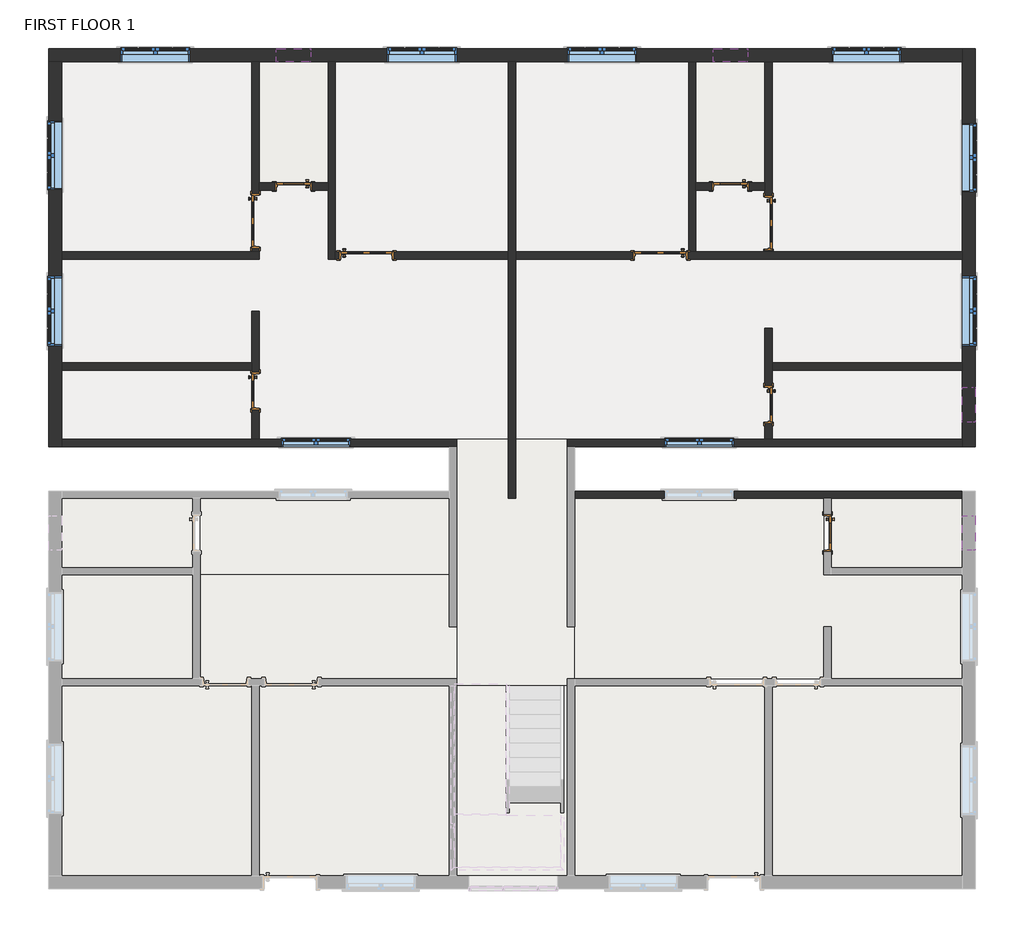
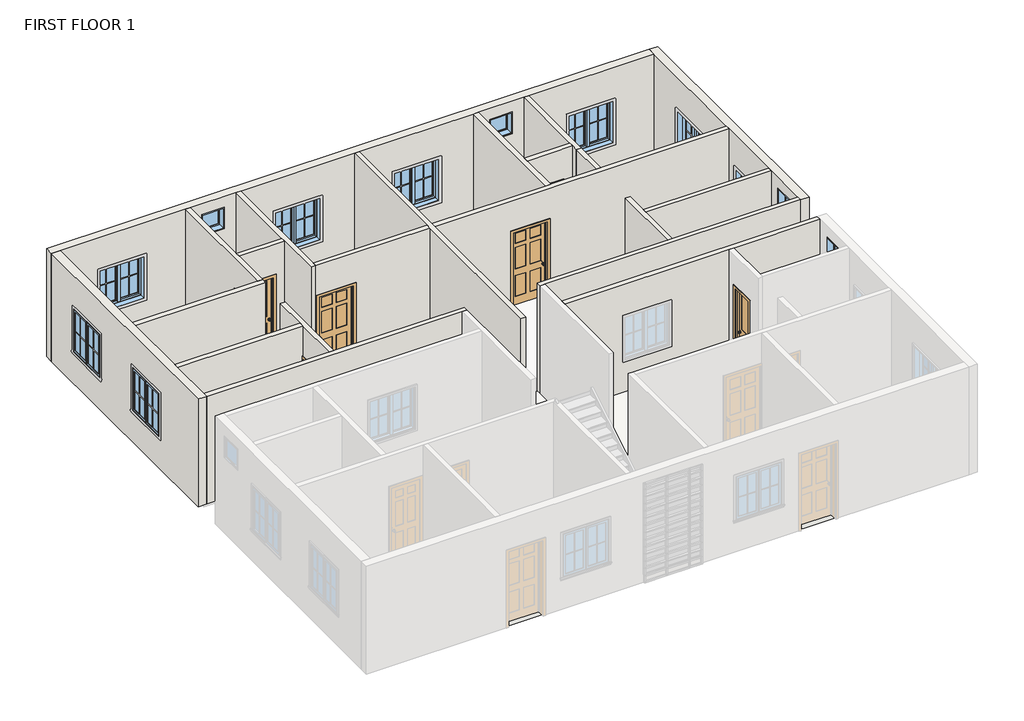
# One storey, part 3 of 4: 21 walls, 14 windows, 9 doors, 9 slabs.
"""IFC4 building model written with IfcOpenShell, lengths in millimetres."""

from ifc_helpers import new_model, si_unit, frame, origin, place, context, project, spatial, polyline, outline, extrude, faceted_brep, transform, mapped, element, save
from components import door_e337afa5, door_596d7c92, door_c610b25b, door_03e3dfb5, window_80340324, window_9200f5ac, window_c2c97eee

model = new_model("IFC4")

# Units and contexts
model_context = context("Model", 3, world=origin())
ifc_project = project(units=[si_unit("LENGTHUNIT", "METRE", prefix="MILLI")], contexts=[model_context])

# Site, building, storey
site = spatial("IfcSite", under=ifc_project)
building = spatial("IfcBuilding", under=site)
storey = spatial("IfcBuildingStorey", under=building, Name="FIRST FLOOR 1", Elevation=3200.4)

# Doors
placement = place(None, origin())
door_shape = door_e337afa5(model_context)
element("IfcDoor", 1, ObjectType="Door-Interior-Single-2_Panel-Wood : 24\" x 84\"", at=placement, inside=storey, context=model_context, shape_type="MappedRepresentation", body=[
    mapped(door_shape, transform((-8112.4137331, 4563.2156164, 3200.4), x_axis=(-1.0, 0.0, 0.0), y_axis=(0.0, -1.0, 0.0), z_axis=(0.0, 0.0, 1.0))),
])
element("IfcDoor", 2, ObjectType="Door-Interior-Single-2_Panel-Wood : 24\" x 84\"", at=placement, inside=storey, context=model_context, shape_type="MappedRepresentation", body=[
    mapped(door_shape, transform((-416.2137331, 4563.2156164, 3200.4), x_axis=(-1.0, 0.0, 0.0), y_axis=(0.0, -1.0, 0.0), z_axis=(0.0, 0.0, 1.0))),
])
element("IfcDoor", 3, ObjectType="Door-Interior-Single-2_Panel-Wood : 24\" x 84\"", at=placement, inside=storey, context=model_context, shape_type="MappedRepresentation", body=[
    mapped(door_shape, transform((-8788.6887331, 953.2406164, 3200.4), x_axis=(0.0, -1.0, 0.0), y_axis=(1.0, 0.0, 0.0), z_axis=(0.0, 0.0, 1.0))),
])
door_2_shape = door_596d7c92(model_context)
element("IfcDoor", 4, ObjectType="Door-Interior-Single-2_Panel-Wood : 24\" x 84\"", at=placement, inside=storey, context=model_context, shape_type="MappedRepresentation", body=[
    mapped(door_2_shape, transform((260.0612669, 711.9406164, 3200.4), x_axis=(0.0, -1.0, 0.0), y_axis=(1.0, 0.0, 0.0), z_axis=(0.0, 0.0, 1.0))),
])
element("IfcDoor", 5, ObjectType="Door-Interior-Single-2_Panel-Wood : 24\" x 84\"", at=placement, inside=storey, context=model_context, shape_type="MappedRepresentation", body=[
    mapped(door_2_shape, transform((1301.4612669, -1548.6593836, 3200.4), x_axis=(0.0, -1.0, 0.0), y_axis=(1.0, 0.0, 0.0), z_axis=(0.0, 0.0, 1.0))),
])
door_3_shape = door_c610b25b(model_context)
element("IfcDoor", 6, ObjectType="Door-Interior-Single-6_Panel-Wood : 36\" x 84\"", at=placement, inside=storey, context=model_context, shape_type="MappedRepresentation", body=[
    mapped(door_3_shape, transform((-8788.6887331, 3950.4406164, 3200.4), x_axis=(0.0, -1.0, 0.0), y_axis=(1.0, 0.0, 0.0), z_axis=(0.0, 0.0, 1.0))),
])
element("IfcDoor", 7, ObjectType="Door-Interior-Single-6_Panel-Wood : 36\" x 84\"", at=placement, inside=storey, context=model_context, shape_type="MappedRepresentation", body=[
    mapped(door_3_shape, transform((-1648.1137331, 3344.0156164, 3200.4), x_axis=(-1.0, 0.0, 0.0), y_axis=(0.0, -1.0, 0.0), z_axis=(0.0, 0.0, 1.0))),
])
door_4_shape = door_03e3dfb5(model_context)
element("IfcDoor", 8, ObjectType="Door-Interior-Single-6_Panel-Wood : 36\" x 84\"", at=placement, inside=storey, context=model_context, shape_type="MappedRepresentation", body=[
    mapped(door_4_shape, transform((-6829.7137331, 3344.0156164, 3200.4), x_axis=(1.0, 0.0, 0.0), y_axis=(0.0, 1.0, 0.0), z_axis=(0.0, 0.0, 1.0))),
])
element("IfcDoor", 9, ObjectType="Door-Interior-Single-6_Panel-Wood : 36\" x 84\"", at=placement, inside=storey, context=model_context, shape_type="MappedRepresentation", body=[
    mapped(door_4_shape, transform((260.0612669, 3912.3406164, 3200.4), x_axis=(0.0, -1.0, 0.0), y_axis=(1.0, 0.0, 0.0), z_axis=(0.0, 0.0, 1.0))),
])

# Slabs
element("IfcSlab", 10, ObjectType="marble tiles", at=placement, inside=storey, context=model_context, shape_type="SweptSolid", body=[
    extrude(outline(polyline([(-9890.4137331, -939.0593836), (-9890.4137331, -2158.2593836), (-12201.8137331, -2158.2593836), (-12201.8137331, -939.0593836), (-9890.4137331, -939.0593836)])), frame((0.0, 0.0, 3048.0), z_axis=(0.0, 0.0, 1.0), x_axis=(1.0, 0.0, 0.0)), (0.0, 0.0, 1.0), 152.4),
    extrude(outline(polyline([(3673.1862669, -2158.2593836), (1361.7862669, -2158.2593836), (1361.7862669, -939.0593836), (3673.1862669, -939.0593836), (3673.1862669, -2158.2593836)])), frame((0.0, 0.0, 3048.0), z_axis=(0.0, 0.0, 1.0), x_axis=(1.0, 0.0, 0.0)), (0.0, 0.0, 1.0), 152.4),
    extrude(outline(polyline([(-7502.8137331, 6758.7281164), (-7502.8137331, 4623.5406164), (-8722.0137331, 4623.5406164), (-8722.0137331, 6758.7281164), (-7502.8137331, 6758.7281164)])), frame((0.0, 0.0, 3048.0), z_axis=(0.0, 0.0, 1.0), x_axis=(1.0, 0.0, 0.0)), (0.0, 0.0, 1.0), 152.4),
    extrude(outline(polyline([(193.3862669, 4623.5406164), (-1025.8137331, 4623.5406164), (-1025.8137331, 6758.7281164), (193.3862669, 6758.7281164), (193.3862669, 4623.5406164)])), frame((0.0, 0.0, 3048.0), z_axis=(0.0, 0.0, 1.0), x_axis=(1.0, 0.0, 0.0)), (0.0, 0.0, 1.0), 152.4),
])
element("IfcSlab", 11, ObjectType="marble tiles", at=placement, inside=storey, context=model_context, shape_type="SweptSolid", body=[
    extrude(outline(polyline([(-5242.2137331, -7593.8593836), (-12201.8137331, -7593.8593836), (-12201.8137331, -2285.2593836), (-5242.2137331, -2285.2593836), (-5242.2137331, -7593.8593836)])), frame((0.0, 0.0, 3048.0), z_axis=(0.0, 0.0, 1.0), x_axis=(1.0, 0.0, 0.0)), (0.0, 0.0, 1.0), 152.4),
])
element("IfcSlab", 12, ObjectType="marble tiles", at=placement, inside=storey, context=model_context, shape_type="SweptSolid", body=[
    extrude(outline(polyline([(-5242.2137331, -2285.2593836), (-9763.4137331, -2285.2593836), (-9763.4137331, -812.0593836), (-5242.2137331, -812.0593836), (-5242.2137331, -2285.2593836)])), frame((0.0, 0.0, 3048.0), z_axis=(0.0, 0.0, 1.0), x_axis=(1.0, 0.0, 0.0)), (0.0, 0.0, 1.0), 152.4),
])
element("IfcSlab", 13, ObjectType="marble tiles", at=placement, inside=storey, context=model_context, shape_type="SweptSolid", body=[
    extrude(outline(polyline([(-3159.4137331, -4241.0593836), (-5242.2137331, -4241.0593836), (-5242.2137331, 102.3406164), (-3159.4137331, 102.3406164), (-3159.4137331, -4241.0593836)])), frame((0.0, 0.0, 3048.0), z_axis=(0.0, 0.0, 1.0), x_axis=(1.0, 0.0, 0.0)), (0.0, 0.0, 1.0), 152.4),
])
element("IfcSlab", 14, ObjectType="marble tiles", at=placement, inside=storey, context=model_context, shape_type="SweptSolid", body=[
    extrude(outline(polyline([(-3286.4137331, -7593.8593836), (-5242.2137331, -7593.8593836), (-5242.2137331, -4241.0593836), (-3286.4137331, -4241.0593836), (-3286.4137331, -7593.8593836)])), frame((0.0, 0.0, 3048.0), z_axis=(0.0, 0.0, 1.0), x_axis=(1.0, 0.0, 0.0)), (0.0, 0.0, 1.0), 152.4),
    extrude(outline(polyline([(193.3862669, -7593.8593836), (-3159.4137331, -7593.8593836), (-3159.4137331, -4241.0593836), (193.3862669, -4241.0593836), (193.3862669, -7593.8593836)])), frame((0.0, 0.0, 3048.0), z_axis=(0.0, 0.0, 1.0), x_axis=(1.0, 0.0, 0.0)), (0.0, 0.0, 1.0), 152.4),
    extrude(outline(polyline([(3673.1862669, -7593.8593836), (320.3862669, -7593.8593836), (320.3862669, -4241.0593836), (3673.1862669, -4241.0593836), (3673.1862669, -7593.8593836)])), frame((0.0, 0.0, 3048.0), z_axis=(0.0, 0.0, 1.0), x_axis=(1.0, 0.0, 0.0)), (0.0, 0.0, 1.0), 152.4),
    extrude(outline(polyline([(1234.7862669, -4114.0593836), (-3159.4137331, -4114.0593836), (-3159.4137331, -939.0593836), (1234.7862669, -939.0593836), (1234.7862669, -2285.2593836), (3673.1862669, -2285.2593836), (3673.1862669, -4114.0593836), (1234.7862669, -4114.0593836)])), frame((0.0, 0.0, 3048.0), z_axis=(0.0, 0.0, 1.0), x_axis=(1.0, 0.0, 0.0)), (0.0, 0.0, 1.0), 152.4),
])
element("IfcSlab", 15, ObjectType="marble tiles", at=placement, inside=storey, context=model_context, shape_type="SweptSolid", body=[
    extrude(outline(polyline([(-5242.2137331, -7593.8593836), (-12201.8137331, -7593.8593836), (-12201.8137331, -2285.2593836), (-5242.2137331, -2285.2593836), (-5242.2137331, -7593.8593836)])), frame((0.0, 0.0, 3048.0), z_axis=(0.0, 0.0, 1.0), x_axis=(1.0, 0.0, 0.0)), (0.0, 0.0, 1.0), 152.4),
])
element("IfcSlab", 16, ObjectType="marble tiles", at=placement, inside=storey, context=model_context, shape_type="SweptSolid", body=[
    extrude(outline(polyline([(-5242.2137331, -2285.2593836), (-9763.4137331, -2285.2593836), (-9763.4137331, -812.0593836), (-5242.2137331, -812.0593836), (-5242.2137331, -2285.2593836)])), frame((0.0, 0.0, 3048.0), z_axis=(0.0, 0.0, 1.0), x_axis=(1.0, 0.0, 0.0)), (0.0, 0.0, 1.0), 152.4),
])
element("IfcSlab", 17, ObjectType="marble tiles", at=placement, inside=storey, context=model_context, shape_type="SweptSolid", body=[
    extrude(outline(polyline([(-3159.4137331, -4241.0593836), (-5242.2137331, -4241.0593836), (-5242.2137331, 102.3406164), (-3159.4137331, 102.3406164), (-3159.4137331, -4241.0593836)])), frame((0.0, 0.0, 3048.0), z_axis=(0.0, 0.0, 1.0), x_axis=(1.0, 0.0, 0.0)), (0.0, 0.0, 1.0), 152.4),
])
element("IfcSlab", 18, ObjectType="marble tiles", at=placement, inside=storey, context=model_context, shape_type="SweptSolid", body=[
    extrude(outline(polyline([(-3286.4137331, -7593.8593836), (-5242.2137331, -7593.8593836), (-5242.2137331, -4241.0593836), (-3286.4137331, -4241.0593836), (-3286.4137331, -7593.8593836)])), frame((0.0, 0.0, 3048.0), z_axis=(0.0, 0.0, 1.0), x_axis=(1.0, 0.0, 0.0)), (0.0, 0.0, 1.0), 152.4),
    extrude(outline(polyline([(193.3862669, -7593.8593836), (-3159.4137331, -7593.8593836), (-3159.4137331, -4241.0593836), (193.3862669, -4241.0593836), (193.3862669, -7593.8593836)])), frame((0.0, 0.0, 3048.0), z_axis=(0.0, 0.0, 1.0), x_axis=(1.0, 0.0, 0.0)), (0.0, 0.0, 1.0), 152.4),
    extrude(outline(polyline([(3673.1862669, -7593.8593836), (320.3862669, -7593.8593836), (320.3862669, -4241.0593836), (3673.1862669, -4241.0593836), (3673.1862669, -7593.8593836)])), frame((0.0, 0.0, 3048.0), z_axis=(0.0, 0.0, 1.0), x_axis=(1.0, 0.0, 0.0)), (0.0, 0.0, 1.0), 152.4),
    extrude(outline(polyline([(1234.7862669, -4114.0593836), (-3159.4137331, -4114.0593836), (-3159.4137331, -939.0593836), (1234.7862669, -939.0593836), (1234.7862669, -2285.2593836), (3673.1862669, -2285.2593836), (3673.1862669, -4114.0593836), (1234.7862669, -4114.0593836)])), frame((0.0, 0.0, 3048.0), z_axis=(0.0, 0.0, 1.0), x_axis=(1.0, 0.0, 0.0)), (0.0, 0.0, 1.0), 152.4),
])

# Walls
element("IfcWall", 19, ObjectType="Inner Wall 5\"", at=placement, inside=storey, context=model_context, shape_type="Brep", body=[
    faceted_brep([(-12201.8137331, -24.6593836, 3200.4), (-5369.2137331, -24.6593836, 3200.4), (-5242.2137331, -24.6593836, 3200.4), (-5242.2137331, -24.6593836, 6248.4), (-5369.2137331, -24.6593836, 6248.4), (-12201.8137331, -24.6593836, 6248.4), (-7109.1137331, -24.6593836, 5334.0), (-7109.1137331, -24.6593836, 4114.8), (-8328.3137331, -24.6593836, 4114.8), (-8328.3137331, -24.6593836, 5334.0), (-12201.8137331, 102.3406164, 3200.4), (-12201.8137331, 102.3406164, 6248.4), (-8849.0137331, 102.3406164, 6248.4), (-8722.0137331, 102.3406164, 6248.4), (-5242.2137331, 102.3406164, 6248.4), (-5242.2137331, 102.3406164, 3200.4), (-8722.0137331, 102.3406164, 3200.4), (-8849.0137331, 102.3406164, 3200.4), (-7109.1137331, 102.3406164, 5334.0), (-8328.3137331, 102.3406164, 5334.0), (-8328.3137331, 102.3406164, 4114.8), (-7109.1137331, 102.3406164, 4114.8)], [[[0, 1, 2, 3, 4, 5], [6, 7, 8, 9]], [[10, 11, 12, 13, 14, 15, 16, 17], [18, 19, 20, 21]], [[2, 1, 0, 10, 17, 16, 15]], [[5, 4, 3, 14, 13, 12, 11]], [[0, 5, 11, 10]], [[3, 2, 15, 14]], [[7, 6, 18, 21]], [[8, 7, 21, 20]], [[9, 8, 20, 19]], [[6, 9, 19, 18]]]),
])
element("IfcWall", 20, ObjectType="Inner Wall 5\"", at=placement, inside=storey, context=model_context, shape_type="Brep", body=[
    faceted_brep([(3673.1862669, 102.3406164, 3200.4), (320.3862669, 102.3406164, 3200.4), (193.3862669, 102.3406164, 3200.4), (-3286.4137331, 102.3406164, 3200.4), (-3286.4137331, 102.3406164, 6248.4), (193.3862669, 102.3406164, 6248.4), (320.3862669, 102.3406164, 6248.4), (3673.1862669, 102.3406164, 6248.4), (-352.7137331, 102.3406164, 5334.0), (-1571.9137331, 102.3406164, 5334.0), (-1571.9137331, 102.3406164, 4114.8), (-352.7137331, 102.3406164, 4114.8), (3673.1862669, -24.6593836, 3200.4), (3673.1862669, -24.6593836, 6248.4), (-3159.4137331, -24.6593836, 6248.4), (-3286.4137331, -24.6593836, 6248.4), (-3286.4137331, -24.6593836, 3200.4), (-3159.4137331, -24.6593836, 3200.4), (-352.7137331, -24.6593836, 5334.0), (-352.7137331, -24.6593836, 4114.8), (-1571.9137331, -24.6593836, 4114.8), (-1571.9137331, -24.6593836, 5334.0)], [[[0, 1, 2, 3, 4, 5, 6, 7], [8, 9, 10, 11]], [[12, 13, 14, 15, 16, 17], [18, 19, 20, 21]], [[3, 2, 1, 0, 12, 17, 16]], [[7, 6, 5, 4, 15, 14, 13]], [[0, 7, 13, 12]], [[4, 3, 16, 15]], [[19, 18, 8, 11]], [[20, 19, 11, 10]], [[21, 20, 10, 9]], [[18, 21, 9, 8]]]),
])
element("IfcWall", 21, ObjectType="Inner Wall 5\"", at=placement, inside=storey, context=model_context, shape_type="Brep", body=[
    faceted_brep([(3673.1862669, -812.0593836, 3200.4), (-3159.4137331, -812.0593836, 3200.4), (-3159.4137331, -812.0593836, 6248.4), (3673.1862669, -812.0593836, 6248.4), (-352.7137331, -812.0593836, 5334.0), (-1571.9137331, -812.0593836, 5334.0), (-1571.9137331, -812.0593836, 4114.8), (-352.7137331, -812.0593836, 4114.8), (3673.1862669, -939.0593836, 3200.4), (3673.1862669, -939.0593836, 6248.4), (1361.7862669, -939.0593836, 6248.4), (1234.7862669, -939.0593836, 6248.4), (-3159.4137331, -939.0593836, 6248.4), (-3159.4137331, -939.0593836, 3200.4), (1234.7862669, -939.0593836, 3200.4), (1361.7862669, -939.0593836, 3200.4), (-352.7137331, -939.0593836, 5334.0), (-352.7137331, -939.0593836, 4114.8), (-1571.9137331, -939.0593836, 4114.8), (-1571.9137331, -939.0593836, 5334.0)], [[[0, 1, 2, 3], [4, 5, 6, 7]], [[8, 9, 10, 11, 12, 13, 14, 15], [16, 17, 18, 19]], [[1, 0, 8, 15, 14, 13]], [[3, 2, 12, 11, 10, 9]], [[0, 3, 9, 8]], [[2, 1, 13, 12]], [[17, 16, 4, 7]], [[18, 17, 7, 6]], [[19, 18, 6, 5]], [[16, 19, 5, 4]]]),
])
element("IfcWall", 22, ObjectType="Inner Wall 5\"", at=placement, inside=storey, context=model_context, shape_type="Brep", body=[
    faceted_brep([(-12201.8137331, 3277.3406164, 3200.4), (-8722.0137331, 3277.3406164, 3200.4), (-8722.0137331, 3277.3406164, 6248.4), (-12201.8137331, 3277.3406164, 6248.4), (-12201.8137331, 3404.3406164, 3200.4), (-12201.8137331, 3404.3406164, 6248.4), (-8849.0137331, 3404.3406164, 6248.4), (-8722.0137331, 3404.3406164, 6248.4), (-8722.0137331, 3404.3406164, 3200.4), (-8849.0137331, 3404.3406164, 3200.4)], [[[0, 1, 2, 3]], [[4, 5, 6, 7, 8, 9]], [[1, 0, 4, 9, 8]], [[3, 2, 7, 6, 5]], [[0, 3, 5, 4]], [[2, 1, 8, 7]]]),
])
element("IfcWall", 23, ObjectType="Inner Wall 5\"", at=placement, inside=storey, context=model_context, shape_type="Brep", body=[
    faceted_brep([(-8722.0137331, 6758.7281164, 6248.4), (-8722.0137331, 4623.5406164, 6248.4), (-8722.0137331, 4496.5406164, 6248.4), (-8722.0137331, 3404.3406164, 6248.4), (-8722.0137331, 3404.3406164, 3200.4), (-8722.0137331, 3467.8406164, 3200.4), (-8722.0137331, 3467.8406164, 5359.4), (-8722.0137331, 4433.0406164, 5359.4), (-8722.0137331, 4433.0406164, 3200.4), (-8722.0137331, 4496.5406164, 3200.4), (-8722.0137331, 4623.5406164, 3200.4), (-8722.0137331, 6758.7281164, 3200.4), (-8849.0137331, 3404.3406164, 6248.4), (-8849.0137331, 6758.7281164, 6248.4), (-8849.0137331, 6758.7281164, 3200.4), (-8849.0137331, 4433.0406164, 3200.4), (-8849.0137331, 4433.0406164, 5359.4), (-8849.0137331, 3467.8406164, 5359.4), (-8849.0137331, 3467.8406164, 3200.4), (-8849.0137331, 3404.3406164, 3200.4)], [[[0, 1, 2, 3, 4, 5, 6, 7, 8, 9, 10, 11]], [[12, 13, 14, 15, 16, 17, 18, 19]], [[4, 19, 18, 5]], [[14, 11, 10, 9, 8, 15]], [[3, 2, 1, 0, 13, 12]], [[4, 3, 12, 19]], [[0, 11, 14, 13]], [[17, 6, 5, 18]], [[6, 17, 16, 7]], [[7, 16, 15, 8]]]),
])
element("IfcWall", 24, ObjectType="Inner Wall 5\"", at=placement, inside=storey, context=model_context, shape_type="SweptSolid", body=[
    extrude(outline(polyline([(6248.4, -7502.8137331), (6248.4, -8722.0137331), (3200.4, -8722.0137331), (3200.4, -8442.6137331), (5359.4, -8442.6137331), (5359.4, -7782.2137331), (3200.4, -7782.2137331), (3200.4, -7502.8137331), (6248.4, -7502.8137331)])), frame((0.0, 4496.5406164, 0.0), z_axis=(0.0, 1.0, 0.0), x_axis=(0.0, 0.0, 1.0)), (0.0, 0.0, 1.0), 127.0),
])
element("IfcWall", 25, ObjectType="Inner Wall 5\"", at=placement, inside=storey, context=model_context, shape_type="Brep", body=[
    faceted_brep([(-7375.8137331, 3277.3406164, 3200.4), (-7375.8137331, 3404.3406164, 3200.4), (-7375.8137331, 6758.7281164, 3200.4), (-7375.8137331, 6758.7281164, 6248.4), (-7375.8137331, 3404.3406164, 6248.4), (-7375.8137331, 3277.3406164, 6248.4), (-7502.8137331, 3277.3406164, 3200.4), (-7502.8137331, 3277.3406164, 6248.4), (-7502.8137331, 4496.5406164, 6248.4), (-7502.8137331, 4623.5406164, 6248.4), (-7502.8137331, 6758.7281164, 6248.4), (-7502.8137331, 6758.7281164, 3200.4), (-7502.8137331, 4623.5406164, 3200.4), (-7502.8137331, 4496.5406164, 3200.4)], [[[0, 1, 2, 3, 4, 5]], [[6, 7, 8, 9, 10, 11, 12, 13]], [[2, 1, 0, 6, 13, 12, 11]], [[5, 4, 3, 10, 9, 8, 7]], [[3, 2, 11, 10]], [[0, 5, 7, 6]]]),
])
element("IfcWall", 26, ObjectType="Inner Wall 5\"", at=placement, inside=storey, context=model_context, shape_type="Brep", body=[
    faceted_brep([(-4327.8137331, 6758.7281164, 3200.4), (-4327.8137331, 3404.3406164, 3200.4), (-4327.8137331, 3277.3406164, 3200.4), (-4327.8137331, -939.0593836, 3200.4), (-4327.8137331, -939.0593836, 6248.4), (-4327.8137331, 3277.3406164, 6248.4), (-4327.8137331, 3404.3406164, 6248.4), (-4327.8137331, 6758.7281164, 6248.4), (-4200.8137331, 6758.7281164, 3200.4), (-4200.8137331, 6758.7281164, 6248.4), (-4200.8137331, 3404.3406164, 6248.4), (-4200.8137331, 3277.3406164, 6248.4), (-4200.8137331, -939.0593836, 6248.4), (-4200.8137331, -939.0593836, 3200.4), (-4200.8137331, 3277.3406164, 3200.4), (-4200.8137331, 3404.3406164, 3200.4)], [[[0, 1, 2, 3, 4, 5, 6, 7]], [[8, 9, 10, 11, 12, 13, 14, 15]], [[3, 2, 1, 0, 8, 15, 14, 13]], [[4, 3, 13, 12]], [[7, 6, 5, 4, 12, 11, 10, 9]], [[0, 7, 9, 8]]]),
])
element("IfcWall", 27, ObjectType="Inner Wall 5\"", at=placement, inside=storey, context=model_context, shape_type="SweptSolid", body=[
    extrude(outline(polyline([(6248.4, -4327.8137331), (6248.4, -7375.8137331), (3200.4, -7375.8137331), (3200.4, -7312.3137331), (5359.4, -7312.3137331), (5359.4, -6347.1137331), (3200.4, -6347.1137331), (3200.4, -4327.8137331), (6248.4, -4327.8137331)])), frame((0.0, 3277.3406164, 0.0), z_axis=(0.0, 1.0, 0.0), x_axis=(0.0, 0.0, 1.0)), (0.0, 0.0, 1.0), 127.0),
])
element("IfcWall", 28, ObjectType="Inner Wall 5\"", at=placement, inside=storey, context=model_context, shape_type="Brep", body=[
    faceted_brep([(3673.1862669, 3277.3406164, 6248.4), (-4200.8137331, 3277.3406164, 6248.4), (-4200.8137331, 3277.3406164, 3200.4), (-2130.7137331, 3277.3406164, 3200.4), (-2130.7137331, 3277.3406164, 5359.4), (-1165.5137331, 3277.3406164, 5359.4), (-1165.5137331, 3277.3406164, 3200.4), (3673.1862669, 3277.3406164, 3200.4), (-4200.8137331, 3404.3406164, 6248.4), (-1152.8137331, 3404.3406164, 6248.4), (-1025.8137331, 3404.3406164, 6248.4), (193.3862669, 3404.3406164, 6248.4), (320.3862669, 3404.3406164, 6248.4), (3673.1862669, 3404.3406164, 6248.4), (3673.1862669, 3404.3406164, 3200.4), (320.3862669, 3404.3406164, 3200.4), (193.3862669, 3404.3406164, 3200.4), (-1025.8137331, 3404.3406164, 3200.4), (-1152.8137331, 3404.3406164, 3200.4), (-1165.5137331, 3404.3406164, 3200.4), (-1165.5137331, 3404.3406164, 5359.4), (-2130.7137331, 3404.3406164, 5359.4), (-2130.7137331, 3404.3406164, 3200.4), (-4200.8137331, 3404.3406164, 3200.4)], [[[0, 1, 2, 3, 4, 5, 6, 7]], [[8, 9, 10, 11, 12, 13, 14, 15, 16, 17, 18, 19, 20, 21, 22, 23]], [[2, 23, 22, 3]], [[14, 7, 6, 19, 18, 17, 16, 15]], [[1, 0, 13, 12, 11, 10, 9, 8]], [[2, 1, 8, 23]], [[0, 7, 14, 13]], [[21, 4, 3, 22]], [[4, 21, 20, 5]], [[5, 20, 19, 6]]]),
])
element("IfcWall", 29, ObjectType="Inner Wall 5\"", at=placement, inside=storey, context=model_context, shape_type="Brep", body=[
    faceted_brep([(-1025.8137331, 3404.3406164, 3200.4), (-1025.8137331, 4496.5406164, 3200.4), (-1025.8137331, 4623.5406164, 3200.4), (-1025.8137331, 6758.7281164, 3200.4), (-1025.8137331, 6758.7281164, 6248.4), (-1025.8137331, 4623.5406164, 6248.4), (-1025.8137331, 4496.5406164, 6248.4), (-1025.8137331, 3404.3406164, 6248.4), (-1152.8137331, 3404.3406164, 3200.4), (-1152.8137331, 3404.3406164, 6248.4), (-1152.8137331, 6758.7281164, 6248.4), (-1152.8137331, 6758.7281164, 3200.4)], [[[0, 1, 2, 3, 4, 5, 6, 7]], [[8, 9, 10, 11]], [[3, 2, 1, 0, 8, 11]], [[7, 6, 5, 4, 10, 9]], [[0, 7, 9, 8]], [[4, 3, 11, 10]]]),
])
element("IfcWall", 30, ObjectType="Inner Wall 5\"", at=placement, inside=storey, context=model_context, shape_type="SweptSolid", body=[
    extrude(outline(polyline([(6248.4, 193.3862669), (6248.4, -1025.8137331), (3200.4, -1025.8137331), (3200.4, -746.4137331), (5359.4, -746.4137331), (5359.4, -86.0137331), (3200.4, -86.0137331), (3200.4, 193.3862669), (6248.4, 193.3862669)])), frame((0.0, 4496.5406164, 0.0), z_axis=(0.0, 1.0, 0.0), x_axis=(0.0, 0.0, 1.0)), (0.0, 0.0, 1.0), 127.0),
])
element("IfcWall", 31, ObjectType="Inner Wall 5\"", at=placement, inside=storey, context=model_context, shape_type="Brep", body=[
    faceted_brep([(320.3862669, 6758.7281164, 6248.4), (320.3862669, 4318.7406164, 6248.4), (320.3862669, 4318.7406164, 5359.4), (320.3862669, 4394.9406164, 5359.4), (320.3862669, 4394.9406164, 3200.4), (320.3862669, 6758.7281164, 3200.4), (193.3862669, 4318.7406164, 6248.4), (193.3862669, 4496.5406164, 6248.4), (193.3862669, 4623.5406164, 6248.4), (193.3862669, 6758.7281164, 6248.4), (193.3862669, 6758.7281164, 3200.4), (193.3862669, 4623.5406164, 3200.4), (193.3862669, 4496.5406164, 3200.4), (193.3862669, 4394.9406164, 3200.4), (193.3862669, 4394.9406164, 5359.4), (193.3862669, 4318.7406164, 5359.4)], [[[0, 1, 2, 3, 4, 5]], [[6, 7, 8, 9, 10, 11, 12, 13, 14, 15]], [[10, 5, 4, 13, 12, 11]], [[1, 0, 9, 8, 7, 6]], [[1, 6, 15, 2]], [[0, 5, 10, 9]], [[14, 3, 2, 15]], [[3, 14, 13, 4]]]),
])
element("IfcWall", 32, ObjectType="Inner Wall 5\"", at=placement, inside=storey, context=model_context, shape_type="SweptSolid", body=[
    extrude(outline(polyline([(320.3862669, 1448.5406164), (3673.1862669, 1448.5406164), (3673.1862669, 1321.5406164), (320.3862669, 1321.5406164), (320.3862669, 1448.5406164)])), frame((0.0, 0.0, 3200.4), z_axis=(0.0, 0.0, 1.0), x_axis=(1.0, 0.0, 0.0)), (0.0, 0.0, 1.0), 3048.0),
])
element("IfcWall", 33, ObjectType="Inner Wall 5\"", at=placement, inside=storey, context=model_context, shape_type="Brep", body=[
    faceted_brep([(193.3862669, 102.3406164, 6248.4), (193.3862669, 2058.1406164, 6248.4), (193.3862669, 2058.1406164, 3200.4), (193.3862669, 1042.1406164, 3200.4), (193.3862669, 1042.1406164, 5359.4), (193.3862669, 381.7406164, 5359.4), (193.3862669, 381.7406164, 3200.4), (193.3862669, 102.3406164, 3200.4), (320.3862669, 2058.1406164, 6248.4), (320.3862669, 1448.5406164, 6248.4), (320.3862669, 1321.5406164, 6248.4), (320.3862669, 102.3406164, 6248.4), (320.3862669, 102.3406164, 3200.4), (320.3862669, 381.7406164, 3200.4), (320.3862669, 381.7406164, 5359.4), (320.3862669, 1042.1406164, 5359.4), (320.3862669, 1042.1406164, 3200.4), (320.3862669, 1321.5406164, 3200.4), (320.3862669, 1448.5406164, 3200.4), (320.3862669, 2058.1406164, 3200.4)], [[[0, 1, 2, 3, 4, 5, 6, 7]], [[8, 9, 10, 11, 12, 13, 14, 15, 16, 17, 18, 19]], [[2, 19, 18, 17, 16, 3]], [[12, 7, 6, 13]], [[1, 0, 11, 10, 9, 8]], [[2, 1, 8, 19]], [[0, 7, 12, 11]], [[5, 14, 13, 6]], [[14, 5, 4, 15]], [[15, 4, 3, 16]]]),
])
element("IfcWall", 34, ObjectType="Inner Wall 5\"", at=placement, inside=storey, context=model_context, shape_type="Brep", body=[
    faceted_brep([(-8722.0137331, 2362.9406164, 3200.4), (-8722.0137331, 2362.9406164, 6248.4), (-8722.0137331, 102.3406164, 6248.4), (-8722.0137331, 102.3406164, 3200.4), (-8722.0137331, 623.0406164, 3200.4), (-8722.0137331, 623.0406164, 5359.4), (-8722.0137331, 1283.4406164, 5359.4), (-8722.0137331, 1283.4406164, 3200.4), (-8849.0137331, 2362.9406164, 6248.4), (-8849.0137331, 2362.9406164, 3200.4), (-8849.0137331, 1448.5406164, 3200.4), (-8849.0137331, 1321.5406164, 3200.4), (-8849.0137331, 1283.4406164, 3200.4), (-8849.0137331, 1283.4406164, 5359.4), (-8849.0137331, 623.0406164, 5359.4), (-8849.0137331, 623.0406164, 3200.4), (-8849.0137331, 102.3406164, 3200.4), (-8849.0137331, 102.3406164, 6248.4), (-8849.0137331, 1321.5406164, 6248.4), (-8849.0137331, 1448.5406164, 6248.4)], [[[0, 1, 2, 3, 4, 5, 6, 7]], [[8, 9, 10, 11, 12, 13, 14, 15, 16, 17, 18, 19]], [[9, 0, 7, 12, 11, 10]], [[3, 16, 15, 4]], [[1, 0, 9, 8]], [[2, 1, 8, 19, 18, 17]], [[3, 2, 17, 16]], [[14, 5, 4, 15]], [[5, 14, 13, 6]], [[6, 13, 12, 7]]]),
])
element("IfcWall", 35, ObjectType="Inner Wall 5\"", at=placement, inside=storey, context=model_context, shape_type="SweptSolid", body=[
    extrude(outline(polyline([(-12201.8137331, 1448.5406164), (-8849.0137331, 1448.5406164), (-8849.0137331, 1321.5406164), (-12201.8137331, 1321.5406164), (-12201.8137331, 1448.5406164)])), frame((0.0, 0.0, 3200.4), z_axis=(0.0, 0.0, 1.0), x_axis=(1.0, 0.0, 0.0)), (0.0, 0.0, 1.0), 3048.0),
])
element("IfcWall", 36, ObjectType="Inner Wall 5\"", at=placement, inside=storey, context=model_context, shape_type="SweptSolid", body=[
    extrude(outline(polyline([(3404.3406164, 6248.4), (4318.7406164, 6248.4), (4318.7406164, 5359.4), (3429.7406164, 5359.4), (3429.7406164, 3200.4), (3404.3406164, 3200.4), (3404.3406164, 6248.4)])), frame((193.3862669, 0.0, 0.0), z_axis=(1.0, 0.0, 0.0), x_axis=(0.0, 1.0, 0.0)), (0.0, 0.0, 1.0), 127.0),
])
element("IfcWall", 37, ObjectType="outer wall 9\"", at=placement, inside=storey, context=model_context, shape_type="Brep", body=[
    faceted_brep([(-12430.4137331, 6758.7281164, 3200.4), (-12201.8137331, 6758.7281164, 3200.4), (-8849.0137331, 6758.7281164, 3200.4), (-8722.0137331, 6758.7281164, 3200.4), (-7502.8137331, 6758.7281164, 3200.4), (-7375.8137331, 6758.7281164, 3200.4), (-4327.8137331, 6758.7281164, 3200.4), (-4200.8137331, 6758.7281164, 3200.4), (-1152.8137331, 6758.7281164, 3200.4), (-1025.8137331, 6758.7281164, 3200.4), (193.3862669, 6758.7281164, 3200.4), (320.3862669, 6758.7281164, 3200.4), (3673.1862669, 6758.7281164, 3200.4), (3673.1862669, 6758.7281164, 6248.4), (320.3862669, 6758.7281164, 6248.4), (193.3862669, 6758.7281164, 6248.4), (-1025.8137331, 6758.7281164, 6248.4), (-1152.8137331, 6758.7281164, 6248.4), (-4200.8137331, 6758.7281164, 6248.4), (-4327.8137331, 6758.7281164, 6248.4), (-7375.8137331, 6758.7281164, 6248.4), (-7502.8137331, 6758.7281164, 6248.4), (-8722.0137331, 6758.7281164, 6248.4), (-8849.0137331, 6758.7281164, 6248.4), (-12201.8137331, 6758.7281164, 6248.4), (-12430.4137331, 6758.7281164, 6248.4), (-9941.2137331, 6758.7281164, 5334.0), (-9941.2137331, 6758.7281164, 4114.8), (-11160.4137331, 6758.7281164, 4114.8), (-11160.4137331, 6758.7281164, 5334.0), (-5242.2137331, 6758.7281164, 5334.0), (-5242.2137331, 6758.7281164, 4114.8), (-6461.4137331, 6758.7281164, 4114.8), (-6461.4137331, 6758.7281164, 5334.0), (-2067.2137331, 6758.7281164, 5334.0), (-2067.2137331, 6758.7281164, 4114.8), (-3286.4137331, 6758.7281164, 4114.8), (-3286.4137331, 6758.7281164, 5334.0), (2593.6862669, 6758.7281164, 5334.0), (2593.6862669, 6758.7281164, 4114.8), (1374.4862669, 6758.7281164, 4114.8), (1374.4862669, 6758.7281164, 5334.0), (-7807.6137331, 6758.7281164, 5943.6), (-7807.6137331, 6758.7281164, 5334.0), (-8417.2137331, 6758.7281164, 5334.0), (-8417.2137331, 6758.7281164, 5943.6), (-111.4137331, 6758.7281164, 5943.6), (-111.4137331, 6758.7281164, 5334.0), (-721.0137331, 6758.7281164, 5334.0), (-721.0137331, 6758.7281164, 5943.6), (-12430.4137331, 6987.3281164, 3200.4), (-12430.4137331, 6987.3281164, 6248.4), (3673.1862669, 6987.3281164, 6248.4), (3673.1862669, 6987.3281164, 3200.4), (-9941.2137331, 6987.3281164, 5334.0), (-11160.4137331, 6987.3281164, 5334.0), (-11160.4137331, 6987.3281164, 4114.8), (-9941.2137331, 6987.3281164, 4114.8), (-5242.2137331, 6987.3281164, 5334.0), (-6461.4137331, 6987.3281164, 5334.0), (-6461.4137331, 6987.3281164, 4114.8), (-5242.2137331, 6987.3281164, 4114.8), (-2067.2137331, 6987.3281164, 5334.0), (-3286.4137331, 6987.3281164, 5334.0), (-3286.4137331, 6987.3281164, 4114.8), (-2067.2137331, 6987.3281164, 4114.8), (2593.6862669, 6987.3281164, 5334.0), (1374.4862669, 6987.3281164, 5334.0), (1374.4862669, 6987.3281164, 4114.8), (2593.6862669, 6987.3281164, 4114.8), (-7807.6137331, 6987.3281164, 5943.6), (-8417.2137331, 6987.3281164, 5943.6), (-8417.2137331, 6987.3281164, 5334.0), (-7807.6137331, 6987.3281164, 5334.0), (-111.4137331, 6987.3281164, 5943.6), (-721.0137331, 6987.3281164, 5943.6), (-721.0137331, 6987.3281164, 5334.0), (-111.4137331, 6987.3281164, 5334.0)], [[[0, 1, 2, 3, 4, 5, 6, 7, 8, 9, 10, 11, 12, 13, 14, 15, 16, 17, 18, 19, 20, 21, 22, 23, 24, 25], [26, 27, 28, 29], [30, 31, 32, 33], [34, 35, 36, 37], [38, 39, 40, 41], [42, 43, 44, 45], [46, 47, 48, 49]], [[50, 51, 52, 53], [54, 55, 56, 57], [58, 59, 60, 61], [62, 63, 64, 65], [66, 67, 68, 69], [70, 71, 72, 73], [74, 75, 76, 77]], [[12, 11, 10, 9, 8, 7, 6, 5, 4, 3, 2, 1, 0, 50, 53]], [[25, 24, 23, 22, 21, 20, 19, 18, 17, 16, 15, 14, 13, 52, 51]], [[0, 25, 51, 50]], [[13, 12, 53, 52]], [[27, 26, 54, 57]], [[28, 27, 57, 56]], [[29, 28, 56, 55]], [[26, 29, 55, 54]], [[31, 30, 58, 61]], [[32, 31, 61, 60]], [[33, 32, 60, 59]], [[30, 33, 59, 58]], [[35, 34, 62, 65]], [[36, 35, 65, 64]], [[37, 36, 64, 63]], [[34, 37, 63, 62]], [[39, 38, 66, 69]], [[40, 39, 69, 68]], [[41, 40, 68, 67]], [[38, 41, 67, 66]], [[43, 42, 70, 73]], [[44, 43, 73, 72]], [[45, 44, 72, 71]], [[42, 45, 71, 70]], [[47, 46, 74, 77]], [[48, 47, 77, 76]], [[49, 48, 76, 75]], [[46, 49, 75, 74]]]),
])
element("IfcWall", 38, ObjectType="outer wall 9\"", at=placement, inside=storey, context=model_context, shape_type="Brep", body=[
    faceted_brep([(-12201.8137331, -24.6593836, 3200.4), (-12201.8137331, 102.3406164, 3200.4), (-12201.8137331, 1321.5406164, 3200.4), (-12201.8137331, 1448.5406164, 3200.4), (-12201.8137331, 3277.3406164, 3200.4), (-12201.8137331, 3404.3406164, 3200.4), (-12201.8137331, 6758.7281164, 3200.4), (-12201.8137331, 6758.7281164, 6248.4), (-12201.8137331, 3404.3406164, 6248.4), (-12201.8137331, 3277.3406164, 6248.4), (-12201.8137331, 1448.5406164, 6248.4), (-12201.8137331, 1321.5406164, 6248.4), (-12201.8137331, 102.3406164, 6248.4), (-12201.8137331, -24.6593836, 6248.4), (-12201.8137331, 2972.5406164, 5334.0), (-12201.8137331, 2972.5406164, 4114.8), (-12201.8137331, 1753.3406164, 4114.8), (-12201.8137331, 1753.3406164, 5334.0), (-12201.8137331, 5716.5343664, 5334.0), (-12201.8137331, 5716.5343664, 4114.8), (-12201.8137331, 4497.3343664, 4114.8), (-12201.8137331, 4497.3343664, 5334.0), (-12430.4137331, -24.6593836, 3200.4), (-12430.4137331, -24.6593836, 6248.4), (-12430.4137331, 6758.7281164, 6248.4), (-12430.4137331, 6758.7281164, 3200.4), (-12430.4137331, 2972.5406164, 5334.0), (-12430.4137331, 1753.3406164, 5334.0), (-12430.4137331, 1753.3406164, 4114.8), (-12430.4137331, 2972.5406164, 4114.8), (-12430.4137331, 5716.5343664, 5334.0), (-12430.4137331, 4497.3343664, 5334.0), (-12430.4137331, 4497.3343664, 4114.8), (-12430.4137331, 5716.5343664, 4114.8)], [[[0, 1, 2, 3, 4, 5, 6, 7, 8, 9, 10, 11, 12, 13], [14, 15, 16, 17], [18, 19, 20, 21]], [[22, 23, 24, 25], [26, 27, 28, 29], [30, 31, 32, 33]], [[6, 5, 4, 3, 2, 1, 0, 22, 25]], [[13, 12, 11, 10, 9, 8, 7, 24, 23]], [[7, 6, 25, 24]], [[0, 13, 23, 22]], [[15, 14, 26, 29]], [[16, 15, 29, 28]], [[17, 16, 28, 27]], [[14, 17, 27, 26]], [[19, 18, 30, 33]], [[20, 19, 33, 32]], [[21, 20, 32, 31]], [[18, 21, 31, 30]]]),
])
element("IfcWall", 39, ObjectType="outer wall 9\"", at=placement, inside=storey, context=model_context, shape_type="Brep", body=[
    faceted_brep([(3673.1862669, 6987.3281164, 3200.4), (3673.1862669, 6758.7281164, 3200.4), (3673.1862669, 3404.3406164, 3200.4), (3673.1862669, 3277.3406164, 3200.4), (3673.1862669, 1448.5406164, 3200.4), (3673.1862669, 1321.5406164, 3200.4), (3673.1862669, 102.3406164, 3200.4), (3673.1862669, -24.6593836, 3200.4), (3673.1862669, -24.6593836, 6248.4), (3673.1862669, 102.3406164, 6248.4), (3673.1862669, 1321.5406164, 6248.4), (3673.1862669, 1448.5406164, 6248.4), (3673.1862669, 3277.3406164, 6248.4), (3673.1862669, 3404.3406164, 6248.4), (3673.1862669, 6758.7281164, 6248.4), (3673.1862669, 6987.3281164, 6248.4), (3673.1862669, 4458.4406164, 5334.0), (3673.1862669, 4458.4406164, 4114.8), (3673.1862669, 5677.6406164, 4114.8), (3673.1862669, 5677.6406164, 5334.0), (3673.1862669, 1753.3406164, 5334.0), (3673.1862669, 1753.3406164, 4114.8), (3673.1862669, 2972.5406164, 4114.8), (3673.1862669, 2972.5406164, 5334.0), (3673.1862669, 407.1406164, 5943.6), (3673.1862669, 407.1406164, 5334.0), (3673.1862669, 1016.7406164, 5334.0), (3673.1862669, 1016.7406164, 5943.6), (3901.7862669, 6987.3281164, 3200.4), (3901.7862669, 6987.3281164, 6248.4), (3901.7862669, -24.6593836, 6248.4), (3901.7862669, -24.6593836, 3200.4), (3901.7862669, 4458.4406164, 5334.0), (3901.7862669, 5677.6406164, 5334.0), (3901.7862669, 5677.6406164, 4114.8), (3901.7862669, 4458.4406164, 4114.8), (3901.7862669, 1753.3406164, 5334.0), (3901.7862669, 2972.5406164, 5334.0), (3901.7862669, 2972.5406164, 4114.8), (3901.7862669, 1753.3406164, 4114.8), (3901.7862669, 407.1406164, 5943.6), (3901.7862669, 1016.7406164, 5943.6), (3901.7862669, 1016.7406164, 5334.0), (3901.7862669, 407.1406164, 5334.0)], [[[0, 1, 2, 3, 4, 5, 6, 7, 8, 9, 10, 11, 12, 13, 14, 15], [16, 17, 18, 19], [20, 21, 22, 23], [24, 25, 26, 27]], [[28, 29, 30, 31], [32, 33, 34, 35], [36, 37, 38, 39], [40, 41, 42, 43]], [[7, 6, 5, 4, 3, 2, 1, 0, 28, 31]], [[15, 14, 13, 12, 11, 10, 9, 8, 30, 29]], [[0, 15, 29, 28]], [[8, 7, 31, 30]], [[17, 16, 32, 35]], [[18, 17, 35, 34]], [[19, 18, 34, 33]], [[16, 19, 33, 32]], [[21, 20, 36, 39]], [[22, 21, 39, 38]], [[23, 22, 38, 37]], [[20, 23, 37, 36]], [[25, 24, 40, 43]], [[26, 25, 43, 42]], [[27, 26, 42, 41]], [[24, 27, 41, 40]]]),
])

# Windows
window_shape = window_80340324(model_context)
element("IfcWindow", 40, ObjectType="Fixed : 24\" x 24\"", at=placement, inside=storey, context=model_context, shape_type="MappedRepresentation", body=[
    mapped(window_shape, transform((3787.4862669, -1586.7593836, 4419.6), x_axis=(0.0, -1.0, 0.0), y_axis=(1.0, 0.0, 0.0), z_axis=(0.0, 0.0, 1.0))),
])
element("IfcWindow", 41, ObjectType="Fixed : 24\" x 24\"", at=placement, inside=storey, context=model_context, shape_type="MappedRepresentation", body=[
    mapped(window_shape, transform((3787.4862669, 673.8406164, 4419.6), x_axis=(0.0, -1.0, 0.0), y_axis=(1.0, 0.0, 0.0), z_axis=(0.0, 0.0, 1.0))),
])
element("IfcWindow", 42, ObjectType="Fixed : 24\" x 24\"", at=placement, inside=storey, context=model_context, shape_type="MappedRepresentation", body=[
    mapped(window_shape, transform((-8074.3137331, 6873.0281164, 4419.6), x_axis=(1.0, 0.0, 0.0), y_axis=(0.0, 1.0, 0.0), z_axis=(0.0, 0.0, 1.0))),
])
element("IfcWindow", 43, ObjectType="Fixed : 24\" x 24\"", at=placement, inside=storey, context=model_context, shape_type="MappedRepresentation", body=[
    mapped(window_shape, transform((-378.1137331, 6873.0281164, 4419.6), x_axis=(1.0, 0.0, 0.0), y_axis=(0.0, 1.0, 0.0), z_axis=(0.0, 0.0, 1.0))),
])
window_2_shape = window_9200f5ac(model_context)
element("IfcWindow", 44, ObjectType="Window-Casement-Double : 48\" x 48\"", at=placement, inside=storey, context=model_context, shape_type="MappedRepresentation", body=[
    mapped(window_2_shape, transform((-12316.1137331, 2362.9406164, 3200.4), x_axis=(0.0, 1.0, 0.0), y_axis=(-1.0, 0.0, 0.0), z_axis=(0.0, 0.0, 1.0))),
])
element("IfcWindow", 45, ObjectType="Window-Casement-Double : 48\" x 48\"", at=placement, inside=storey, context=model_context, shape_type="MappedRepresentation", body=[
    mapped(window_2_shape, transform((-12316.1137331, 5106.9343664, 3200.4), x_axis=(0.0, 1.0, 0.0), y_axis=(-1.0, 0.0, 0.0), z_axis=(0.0, 0.0, 1.0))),
])
element("IfcWindow", 46, ObjectType="Window-Casement-Double : 48\" x 48\"", at=placement, inside=storey, context=model_context, shape_type="MappedRepresentation", body=[
    mapped(window_2_shape, transform((-10550.8137331, 6873.0281164, 3200.4), x_axis=(1.0, 0.0, 0.0), y_axis=(0.0, 1.0, 0.0), z_axis=(0.0, 0.0, 1.0))),
])
element("IfcWindow", 47, ObjectType="Window-Casement-Double : 48\" x 48\"", at=placement, inside=storey, context=model_context, shape_type="MappedRepresentation", body=[
    mapped(window_2_shape, transform((-5851.8137331, 6873.0281164, 3200.4), x_axis=(1.0, 0.0, 0.0), y_axis=(0.0, 1.0, 0.0), z_axis=(0.0, 0.0, 1.0))),
])
element("IfcWindow", 48, ObjectType="Window-Casement-Double : 48\" x 48\"", at=placement, inside=storey, context=model_context, shape_type="MappedRepresentation", body=[
    mapped(window_2_shape, transform((-2676.8137331, 6873.0281164, 3200.4), x_axis=(1.0, 0.0, 0.0), y_axis=(0.0, 1.0, 0.0), z_axis=(0.0, 0.0, 1.0))),
])
element("IfcWindow", 49, ObjectType="Window-Casement-Double : 48\" x 48\"", at=placement, inside=storey, context=model_context, shape_type="MappedRepresentation", body=[
    mapped(window_2_shape, transform((1984.0862669, 6873.0281164, 3200.4), x_axis=(1.0, 0.0, 0.0), y_axis=(0.0, 1.0, 0.0), z_axis=(0.0, 0.0, 1.0))),
])
element("IfcWindow", 50, ObjectType="Window-Casement-Double : 48\" x 48\"", at=placement, inside=storey, context=model_context, shape_type="MappedRepresentation", body=[
    mapped(window_2_shape, transform((3787.4862669, 5068.0406164, 3200.4), x_axis=(0.0, -1.0, 0.0), y_axis=(1.0, 0.0, 0.0), z_axis=(0.0, 0.0, 1.0))),
])
element("IfcWindow", 51, ObjectType="Window-Casement-Double : 48\" x 48\"", at=placement, inside=storey, context=model_context, shape_type="MappedRepresentation", body=[
    mapped(window_2_shape, transform((3787.4862669, 2362.9406164, 3200.4), x_axis=(0.0, -1.0, 0.0), y_axis=(1.0, 0.0, 0.0), z_axis=(0.0, 0.0, 1.0))),
])
window_3_shape = window_c2c97eee(model_context)
element("IfcWindow", 52, ObjectType="Window-Casement-Double : 48\" x 48\"", at=placement, inside=storey, context=model_context, shape_type="MappedRepresentation", body=[
    mapped(window_3_shape, transform((-7718.7137331, 38.8406164, 3200.4), x_axis=(1.0, 0.0, 0.0), y_axis=(0.0, 1.0, 0.0), z_axis=(0.0, 0.0, 1.0))),
])
element("IfcWindow", 53, ObjectType="Window-Casement-Double : 48\" x 48\"", at=placement, inside=storey, context=model_context, shape_type="MappedRepresentation", body=[
    mapped(window_3_shape, transform((-962.3137331, 38.8406164, 3200.4), x_axis=(1.0, 0.0, 0.0), y_axis=(0.0, 1.0, 0.0), z_axis=(0.0, 0.0, 1.0))),
])

save(model, "model.ifc")

# Revit data of these elements
# Type "Door-Interior-Single-2_Panel-Wood : 24\" x 84\""
#   Type Mark = "10"
#   Assembly Code = "C1020300"
#   Analytic Construction = "Wooden"
#   Top Rail = 0' - 4 11/16"
#   Thickness = 0' - 1 3/8"
#   Thermal Resistance (R) = 2.5876 (h·ft²·°F)/BTU
#   Swing Angle [instance default] = 90.00°
#   Stiles = 0' - 4 3/4"
#   Rough Width = 2' - 2"
#   Rough Height = 7' - 1"
#   Lock Rail = 0' - 7 1/2"
#   Height = 7' - 0"
#   Width = 2' - 0"
#   Heat Transfer Coefficient (U) = 0.3865 BTU/(h·ft²·°F)
#   Bottom Rail = 0' - 9 1/8"
#   Trim Material = Cherry
#   Panel Material = Cherry
#   Frame Material = Cherry
#   Door Handle Material = Aluminum
#   Visual Light Transmittance = 0
#   Solar Heat Gain Coefficient = 0
#   Wall Closure = (empty or 0)
#   Function = (empty or 0)
# Type "Door-Interior-Single-6_Panel-Wood : 36\" x 84\""
#   Type Mark = "8"
#   Assembly Code = "C1020300"
#   Analytic Construction = "Wooden"
#   Top Rail = 0' - 4 11/16"
#   Top Panel = 0' - 11"
#   Thickness = 0' - 1 3/8"
#   Thermal Resistance (R) = 2.5876 (h·ft²·°F)/BTU
#   Swing Angle [instance default] = 90.00°
#   Stiles = 0' - 4 3/4"
#   Rough Width = 3' - 2"
#   Rough Height = 7' - 1"
#   Mullion = 0' - 4 1/2"
#   Lock Rail = 0' - 7 1/2"
#   Intermediate Rail = 0' - 4 1/2"
#   Height = 7' - 0"
#   Width = 3' - 0"
#   Heat Transfer Coefficient (U) = 0.3865 BTU/(h·ft²·°F)
#   Bottom Rail = 0' - 9 1/8"
#   Trim Material = Cherry
#   Panel Material = Cherry
#   Frame Material = Cherry
#   Door Handle Material = Aluminum
#   Visual Light Transmittance = 0
#   Solar Heat Gain Coefficient = 0
#   Wall Closure = (empty or 0)
#   Function = (empty or 0)
# Type "marble tiles"
#   Assembly Code = "B1010"
#   Function = 0
#   Layers, outside or top first: 0' - 6" "marble flooring" (function 1)
# Type "Inner Wall 5\""
#   Assembly Code = "B2010"
#   Layers, outside or top first: 0' - 5" "wall paint" (function 1)
# Type "outer wall 9\""
#   Assembly Code = "B2010"
#   Layers, outside or top first: 0' - 9" "wall paint" (function 1)
# Type "Fixed : 24\" x 24\""
#   Type Mark = "3"
#   Construction Type Id = "GSP4R"
#   Assembly Code = "B2020100"
#   Analytic Construction = "1/8 in Pilkington single glazing"
#   Visual Light Transmittance = 0.9
#   Solar Heat Gain Coefficient = 0.78
#   Heat Transfer Coefficient (U) = 0.6496 BTU/(h·ft²·°F)
#   Height = 2' - 0"
#   Default Sill Height = 3' - 0"
#   Width = 2' - 0"
#   Window Inset = 0' - 0 3/4"
#   Define Thermal Properties by = 1
#   Define Thermal Properties by = 1
#   Glass Pane Material = Glass
#   Sash Material = Sash
#   Wall Closure = (empty or 0)
# Type "Window-Casement-Double : 48\" x 48\""
#   Type Mark = "18"
#   Fire Rating = "0.5h"
#   Assembly Code = "B2020100"
#   Analytic Construction = "Double glazing - domestic"
#   Frame Extension [instance default] = 0' - 0 1/4"
#   Window Inset [instance default] = 0' - 0"
#   Wall Thickness [instance default] = 0' - 6"
#   Interior Wall Closure [instance default] = 0' - 2 1/4"
#   Half Width = 2' - 0"
#   Visual Light Transmittance = 0.81
#   Thermal Resistance (R) = 1.8146 (h·ft²·°F)/BTU
#   Solar Heat Gain Coefficient = 0.76
#   Rough Width = 4' - 0 1/2"
#   Rough Height = 4' - 0 1/2"
#   Height = 4' - 0"
#   Heat Transfer Coefficient (U) = 0.5511 BTU/(h·ft²·°F)
#   Exterior Wall Closure [instance default] = 0' - 1 1/4"
#   Extension Jamb [instance default] = 0' - 2 1/4"
#   Default Sill Height = 3' - 0"
#   Width = 4' - 0"
#   Muntin Visibility = yes
#   Interior Trim Visibility [instance default] = yes
#   Exterior Trim Visibility [instance default] = yes
#   Extension Jamb Visibility [instance default] = yes
#   Interior Trim Material = Wood - Stained
#   Muntin Pattern = Muntin Pattern_2x2 : Muntin Pattern_2x2
#   Interior Trim = Trim-Window-Interior-Flat : Picture Frame
#   Interior Frame Material = Wood - Stained
#   Glass Panel Material = Glass
#   Exterior Trim Material = Clad - White
#   Exterior Trim = Trim-Window-Exterior-Flat : with Sill
#   Exterior Frame Material = Clad - White
#   Wall Closure = (empty or 0)
# Elements 1, 2, 3, 4, 5 (IfcDoor, "Door-Interior-Single-2_Panel-Wood : 24\" x 84\"")
#   Swing Angle = 90.00°
#   Phase Created = New Construction
#   Materials on its faces: "Cherry", "Aluminum"
# Elements 6, 7, 8, 9 (IfcDoor, "Door-Interior-Single-6_Panel-Wood : 36\" x 84\"")
#   Swing Angle = 90.00°
#   Phase Created = New Construction
#   Materials on its faces: "Cherry", "Aluminum"
# Elements 10, 11, 12, 13, 14, 15, 16, 17, 18 (IfcSlab, "marble tiles")
#   Height Offset From Level = 0' - 0"
#   Phase Created = New Construction
#   Materials on its faces: "marble flooring"
# Elements 19, 20, 21 (IfcWall, "Inner Wall 5\"")
#   Top Offset = 0' - 0"
#   Base Offset = 0' - 0"
#   Unconnected Height = 10' - 0"
#   wall height = 10' - 0"
#   Phase Created = New Construction
#   Base Constraint = FIRST FLOOR 1
#   Materials on its faces: "wall paint", "Clad - White"
# Elements 22, 23, 24, 25, 26, 27, 28, 29, 30, 31, 32, 33, 34, 35, 36 (IfcWall, "Inner Wall 5\"")
#   Top Offset = 0' - 0"
#   Base Offset = 0' - 0"
#   Unconnected Height = 10' - 0"
#   wall height = 10' - 0"
#   Phase Created = New Construction
#   Base Constraint = FIRST FLOOR 1
#   Materials on its faces: "wall paint"
# Elements 37, 38, 39 (IfcWall, "outer wall 9\"")
#   Top Offset = 0' - 0"
#   Base Offset = 0' - 0"
#   Unconnected Height = 10' - 0"
#   wall height = 10' - 0"
#   Phase Created = New Construction
#   Base Constraint = FIRST FLOOR 1
#   Materials on its faces: "wall paint", "Clad - White"
# Element 40 (IfcWindow, "Fixed : 24\" x 24\"")
#   Mark = "42"
#   Phase Created = New Construction
#   Materials on its faces: "Sash", "Glass"
# Element 41 (IfcWindow, "Fixed : 24\" x 24\"")
#   Mark = "43"
#   Phase Created = New Construction
#   Materials on its faces: "Sash", "Glass"
# Element 42 (IfcWindow, "Fixed : 24\" x 24\"")
#   Mark = "45"
#   Phase Created = New Construction
#   Materials on its faces: "Sash", "Glass"
# Element 43 (IfcWindow, "Fixed : 24\" x 24\"")
#   Mark = "46"
#   Phase Created = New Construction
#   Materials on its faces: "Sash", "Glass"
# Element 44 (IfcWindow, "Window-Casement-Double : 48\" x 48\"")
#   Mark = "24"
#   Window Inset = 0' - 0"
#   Interior Wall Closure = 0' - 2 1/4"
#   Frame Extension = 0' - 0 1/4"
#   Exterior Wall Closure = 0' - 1 1/4"
#   Interior Trim Visibility = yes
#   Exterior Trim Visibility = yes
#   Phase Created = New Construction
#   Materials on its faces: "Wood - Stained", "Glass", "Clad - White"
# Element 45 (IfcWindow, "Window-Casement-Double : 48\" x 48\"")
#   Mark = "25"
#   Window Inset = 0' - 0"
#   Interior Wall Closure = 0' - 2 1/4"
#   Frame Extension = 0' - 0 1/4"
#   Exterior Wall Closure = 0' - 1 1/4"
#   Interior Trim Visibility = yes
#   Exterior Trim Visibility = yes
#   Phase Created = New Construction
#   Materials on its faces: "Wood - Stained", "Glass", "Clad - White"
# Element 46 (IfcWindow, "Window-Casement-Double : 48\" x 48\"")
#   Mark = "26"
#   Window Inset = 0' - 0"
#   Interior Wall Closure = 0' - 2 1/4"
#   Frame Extension = 0' - 0 1/4"
#   Exterior Wall Closure = 0' - 1 1/4"
#   Interior Trim Visibility = yes
#   Exterior Trim Visibility = yes
#   Phase Created = New Construction
#   Materials on its faces: "Wood - Stained", "Glass", "Clad - White"
# Element 47 (IfcWindow, "Window-Casement-Double : 48\" x 48\"")
#   Mark = "27"
#   Window Inset = 0' - 0"
#   Interior Wall Closure = 0' - 2 1/4"
#   Frame Extension = 0' - 0 1/4"
#   Exterior Wall Closure = 0' - 1 1/4"
#   Interior Trim Visibility = yes
#   Exterior Trim Visibility = yes
#   Phase Created = New Construction
#   Materials on its faces: "Wood - Stained", "Glass", "Clad - White"
# Element 48 (IfcWindow, "Window-Casement-Double : 48\" x 48\"")
#   Mark = "28"
#   Window Inset = 0' - 0"
#   Interior Wall Closure = 0' - 2 1/4"
#   Frame Extension = 0' - 0 1/4"
#   Exterior Wall Closure = 0' - 1 1/4"
#   Interior Trim Visibility = yes
#   Exterior Trim Visibility = yes
#   Phase Created = New Construction
#   Materials on its faces: "Wood - Stained", "Glass", "Clad - White"
# Element 49 (IfcWindow, "Window-Casement-Double : 48\" x 48\"")
#   Mark = "29"
#   Window Inset = 0' - 0"
#   Interior Wall Closure = 0' - 2 1/4"
#   Frame Extension = 0' - 0 1/4"
#   Exterior Wall Closure = 0' - 1 1/4"
#   Interior Trim Visibility = yes
#   Exterior Trim Visibility = yes
#   Phase Created = New Construction
#   Materials on its faces: "Wood - Stained", "Glass", "Clad - White"
# Element 50 (IfcWindow, "Window-Casement-Double : 48\" x 48\"")
#   Mark = "30"
#   Window Inset = 0' - 0"
#   Interior Wall Closure = 0' - 2 1/4"
#   Frame Extension = 0' - 0 1/4"
#   Exterior Wall Closure = 0' - 1 1/4"
#   Interior Trim Visibility = yes
#   Exterior Trim Visibility = yes
#   Phase Created = New Construction
#   Materials on its faces: "Wood - Stained", "Glass", "Clad - White"
# Element 51 (IfcWindow, "Window-Casement-Double : 48\" x 48\"")
#   Mark = "31"
#   Window Inset = 0' - 0"
#   Interior Wall Closure = 0' - 2 1/4"
#   Frame Extension = 0' - 0 1/4"
#   Exterior Wall Closure = 0' - 1 1/4"
#   Interior Trim Visibility = yes
#   Exterior Trim Visibility = yes
#   Phase Created = New Construction
#   Materials on its faces: "Wood - Stained", "Glass", "Clad - White"
# Element 52 (IfcWindow, "Window-Casement-Double : 48\" x 48\"")
#   Mark = "39"
#   Window Inset = 0' - 0"
#   Interior Wall Closure = 0' - 2 1/4"
#   Frame Extension = 0' - 0 1/4"
#   Exterior Wall Closure = 0' - 1 1/4"
#   Interior Trim Visibility = yes
#   Exterior Trim Visibility = yes
#   Phase Created = New Construction
#   Materials on its faces: "Wood - Stained", "Glass", "Clad - White"
# Element 53 (IfcWindow, "Window-Casement-Double : 48\" x 48\"")
#   Mark = "41"
#   Window Inset = 0' - 0"
#   Interior Wall Closure = 0' - 2 1/4"
#   Frame Extension = 0' - 0 1/4"
#   Exterior Wall Closure = 0' - 1 1/4"
#   Interior Trim Visibility = yes
#   Exterior Trim Visibility = yes
#   Phase Created = New Construction
#   Materials on its faces: "Wood - Stained", "Glass", "Clad - White"
# Materials
#   "Cherry": class "Wood", colour RGB 226 177 128, transparency 0, Description = "Prunus Serotina", Cost = 0
#   "Aluminum": class "Metal", colour RGB 247 247 247, transparency 0, Description = "Aluminum 6061", Cost = 0
#   "marble flooring": class "Generic", colour RGB 120 120 120, transparency 0, Cost = 0
#   "wall paint": class "Generic", colour RGB 120 120 120, transparency 0, Cost = 0
#   "Glass": class "Glass", colour RGB 0 128 192, transparency 0.75, Description = "Soda Lime Glass", Cost = 0
#   "Sash": class "Wood", colour RGB 224 178 126, transparency 0, Cost = 0
#   "Wood - Stained": class "Wood", colour RGB 224 178 126, transparency 0, Cost = 0
#   "Clad - White": class "Wood", colour RGB 242 242 238, transparency 0, Cost = 0
